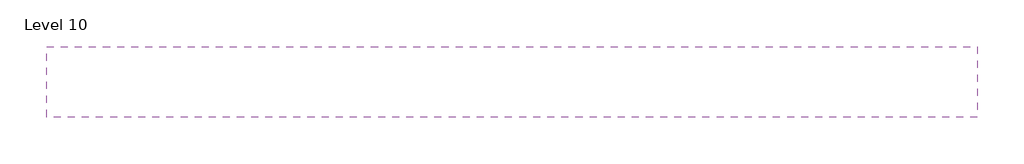
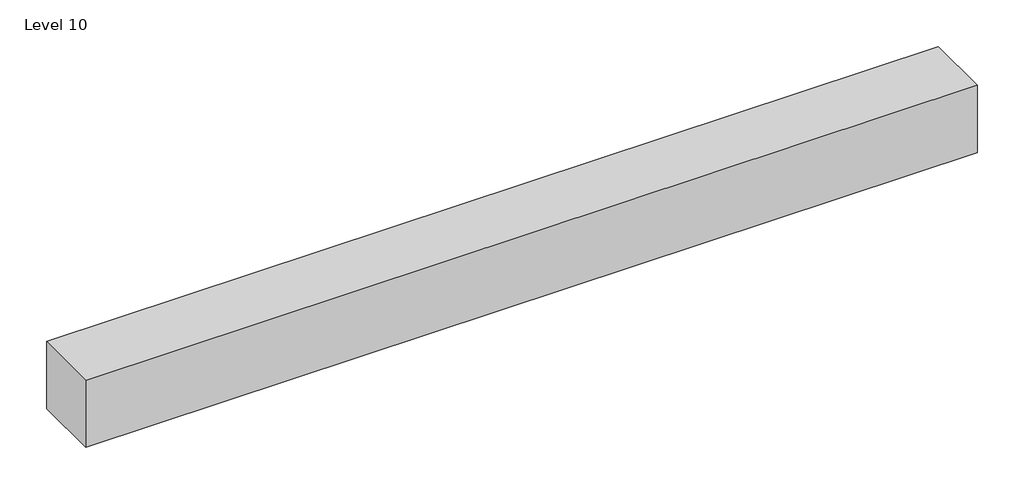
# One storey: 1 proxy.
"""IFC4 building model written with IfcOpenShell, lengths in millimetres."""

from ifc_helpers import new_model, si_unit, origin, place, context, project, spatial, transform, mapped, element, save
from components import generic_models_5_generic_models_5_43fa52cd

model = new_model("IFC4")

# Units and contexts
model_context = context("Model", 3, world=origin())
ifc_project = project(units=[si_unit("LENGTHUNIT", "METRE", prefix="MILLI")], contexts=[model_context])

# Site, building, storey
site = spatial("IfcSite", under=ifc_project)
building = spatial("IfcBuilding", under=site)
storey = spatial("IfcBuildingStorey", under=building, Name="Level 10", Elevation=9829.8)

# Proxy
placement = place(None, origin())
generic_models_5_generic_models_5_shape = generic_models_5_generic_models_5_43fa52cd(model_context)
element("IfcBuildingElementProxy", 1, Name="Generic Models 5 : Generic Models 5", ObjectType="Generic Models 5 : Generic Models 5", at=placement, inside=storey, context=model_context, shape_type="MappedRepresentation", body=[
    mapped(generic_models_5_generic_models_5_shape, transform((0.0, 0.0, 0.0), x_axis=(1.0, 0.0, 0.0), y_axis=(0.0, 1.0, 0.0), z_axis=(0.0, 0.0, 1.0))),
])

save(model, "model.ifc")

# Revit data of these elements
# Element 1 (IfcBuildingElementProxy, "Generic Models 5 : Generic Models 5")
#   Phase Created = New Construction
